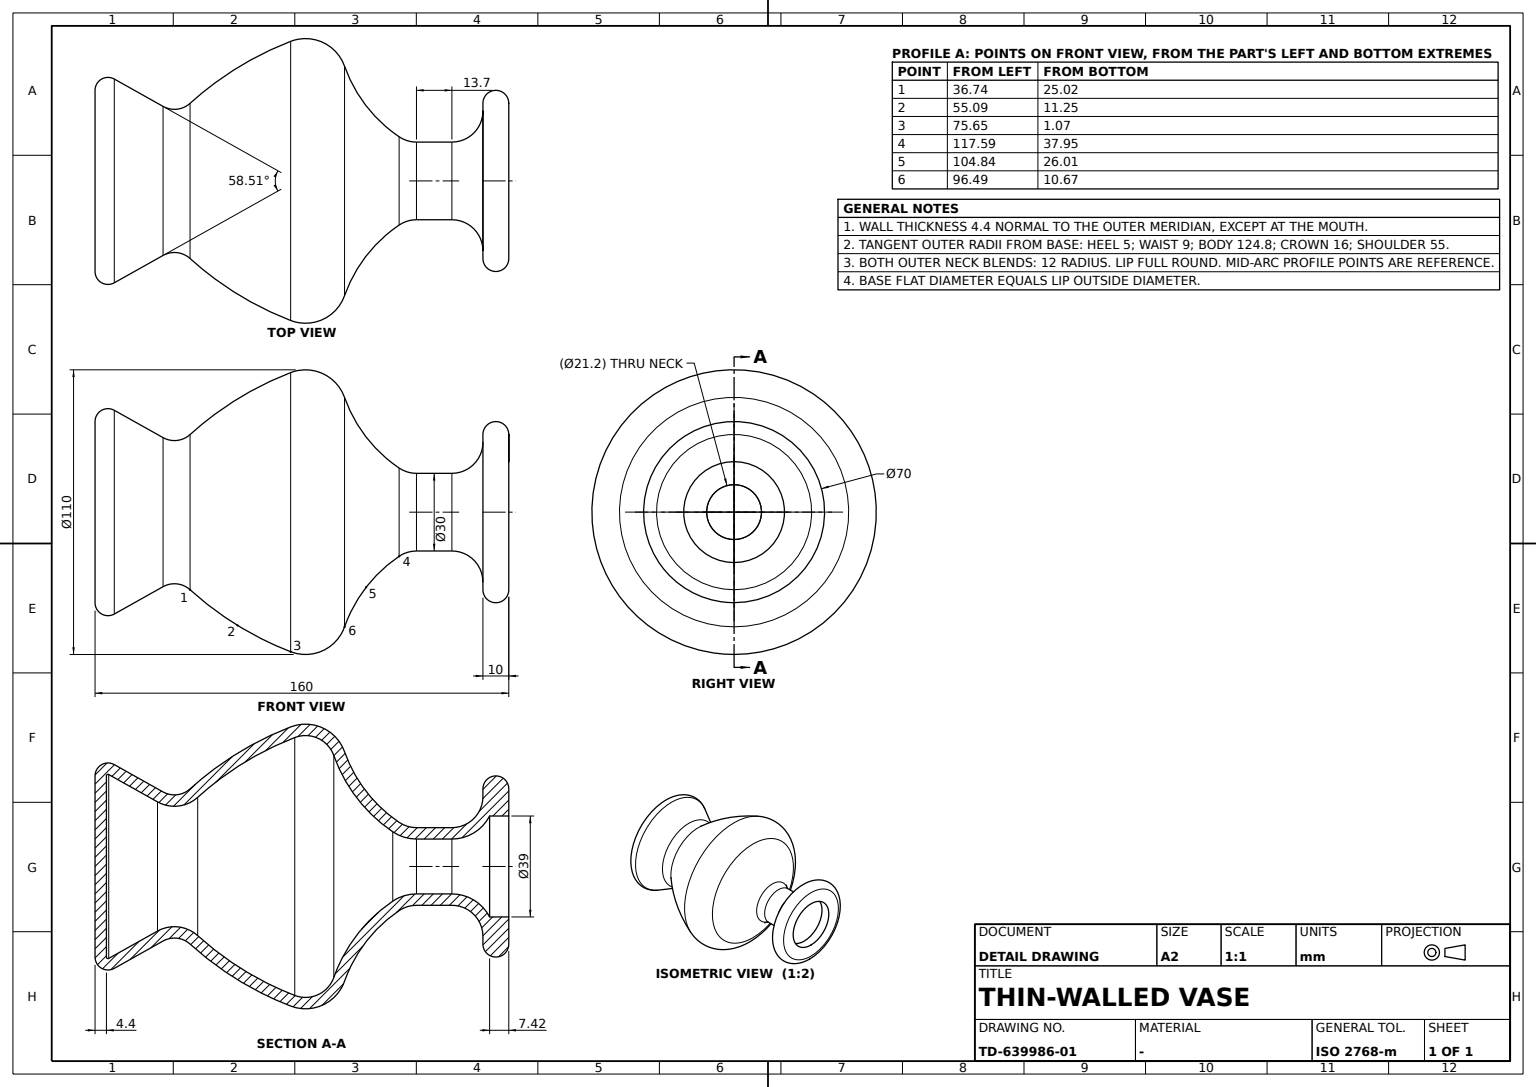
CATIA V5 part; units mm, degrees
sketch "Sketch1" plane through (0, 0, 0) normal (0, 1, 0) x (-1, 0, 0)
  line L0 (0, 0) -> (35, 0)
  arc A0 (35, 0) -> (39.3622, 7.4437) centre (35, 5) ccw
  point P0 (35, 5)
  line L1 (39.3622, 7.4437) -> (28.7981, 26.3014)
  arc A1 (28.7981, 26.3014) -> (29.979, 36.7413) centre (36.65, 30.7) cw
  point P1 (36.65, 30.7)
  point P2 (29.979, 36.7413)
  arc A2 (29.979, 36.7413) -> (53.9303, 75.6479) centre (-62.526, 120.514) ccw
  point P3 (-62.526, 120.514)
  point P4 (29.979, 36.7413)
  arc A3 (53.9303, 75.6479) -> (44.3292, 96.4864) centre (39, 81.4) ccw
  point P5 (39, 81.4)
  arc A4 (44.3292, 96.4864) -> (17.0517, 117.5895) centre (62.6481, 148.346) cw
  point P6 (62.6481, 148.346)
  arc A5 (17.0517, 117.5895) -> (15, 124.3) centre (27, 124.3) cw
  point P7 (27, 124.3)
  point P8 (15, 124.3)
  point P9 (15, 124.3)
  line L2 (15, 124.3) -> (15, 138)
  point P10 (15, 138)
  arc A6 (15, 138) -> (27, 150) centre (27, 138) cw
  point P11 (27, 138)
  line L3 (0, 155) -> (30, 155) construction
  point P12 (0, 155)
  line L4 (30, 150) -> (27, 150)
  arc A7 (30, 160) -> (30, 150) centre (30, 155) cw
  point P13 (0, 160)
  line L5 (0, 160) -> (0, 160) construction
  line L6 (0, 0) -> (0, 155) construction
  line L7 (0, 4.4) -> (35, 4.4)
  line L8 (0, 0) -> (0, 4.4) construction
  line L9 (35, 0) -> (35, 4.4) construction
  arc A8 (35, 4.4) -> (35.5235, 5.2932) centre (35, 5) ccw
  line L10 (35, 0) -> (35, 4.4) construction
  line L11 (39.3622, 7.4437) -> (35.5235, 5.2932) construction
  line L12 (35.5235, 5.2932) -> (24.9594, 24.151)
  line L13 (39.3622, 7.4437) -> (35.5235, 5.2932) construction
  line L14 (28.7981, 26.3014) -> (24.9594, 24.151) construction
  arc A9 (26.7176, 39.6948) -> (24.9594, 24.151) centre (36.65, 30.7) ccw
  line L15 (29.979, 36.7413) -> (26.7176, 39.6948) construction
  line L16 (28.7981, 26.3014) -> (24.9594, 24.151) construction
  arc A10 (26.7176, 39.6948) -> (49.8245, 77.2298) centre (-62.526, 120.514) ccw
  line L17 (29.979, 36.7413) -> (26.7176, 39.6948) construction
  line L18 (53.9303, 75.6479) -> (49.8245, 77.2298) construction
  arc A11 (49.8245, 77.2298) -> (42.8636, 92.3377) centre (39, 81.4) ccw
  line L19 (53.9303, 75.6479) -> (49.8245, 77.2298) construction
  line L20 (44.3292, 96.4864) -> (42.8636, 92.3377) construction
  arc A12 (13.404, 115.129) -> (42.8636, 92.3377) centre (62.6481, 148.346) ccw
  line L21 (17.0517, 117.5895) -> (13.404, 115.129) construction
  line L22 (44.3292, 96.4864) -> (42.8636, 92.3377) construction
  arc A13 (10.6, 124.3) -> (13.404, 115.129) centre (27, 124.3) ccw
  line L23 (15, 124.3) -> (10.6, 124.3) construction
  line L24 (17.0517, 117.5895) -> (13.404, 115.129) construction
  line L25 (10.6, 124.3) -> (10.6, 138)
  line L26 (15, 124.3) -> (10.6, 124.3) construction
  line L27 (15, 138) -> (10.6, 138) construction
  arc A14 (19.5, 152.5846) -> (10.6, 138) centre (27, 138) ccw
  line L28 (27, 150) -> (27, 154.4) construction
  line L29 (15, 138) -> (10.6, 138) construction
  line L30 (0, 160) -> (19.5, 160) construction
  point P14 (19.5, 160)
  line L31 (19.5, 160) -> (30, 160)
  line L32 (19.5, 160) -> (19.5, 152.5846)
  line L33 (0, 0) -> (0, 4.4)
  dimension "radius A0" = 5
  dimension "radius A1" = 9
  dimension "distance A1 y axis" = 27.65
  dimension "length L0" = 35
  dimension "distance A1 L0" = 21.7
  dimension "radius A2" = 124.8
  dimension "radius A3" = 16
  dimension "distance P5 A1 y axis" = 59.7
  dimension "distance A3 y axis" = 55
  dimension "length L2" = 13.7
  dimension "radius A5" = 12
  dimension "radius A4" = 55
  dimension "distance y axis P10" = 15
  dimension "radius A6" = 12
  dimension "distance A7 L5" = 35
  dimension "radius A7" = 5
  dimension "distance L0 L7" = 4.4
  dimension "distance A0 A8" = 4.4
  dimension "distance L1 L12" = 4.4
  dimension "distance A1 A9" = 4.4
  dimension "distance A2 A10" = 4.4
  dimension "distance A3 A11" = 4.4
  dimension "distance A4 A12" = 4.4
  dimension "distance A5 A13" = 4.4
  dimension "distance L2 L25" = 4.4
  dimension "distance A6 A14" = 4.4
  dimension "distance A7 P14 x axis" = 15.5
  dimension "distance L31 L0" = 160
  constraint horizontal L0 x-axis
  constraint horizontal L3 x-axis
  constraint horizontal L4 x-axis
  constraint horizontal L31 x-axis
  constraint tangency A0 L0
  constraint tangency L1 A0
  constraint tangency A1 L1
  constraint tangency A3 A2
  constraint tangency A2 A1
  constraint tangency A5 L2
  constraint tangency A4 A3
  constraint tangency A4 A5
  constraint tangency A6 L2
  constraint tangency A7 L4
  constraint tangency A6 L4
  constraint tangency L30 A7
  constraint tangency L31 A7
  constraint coincidence P2 P4
  constraint coincidence P9 A5
  constraint coincidence P9 P8
  constraint coincidence P12 y-axis
  constraint coincidence P13 L5
  constraint coincidence P13 y-axis
  constraint coincidence L10 P0
  constraint coincidence L11 P0
  constraint coincidence L15 P1
  constraint coincidence L16 P1
  constraint coincidence L17 P3
  constraint coincidence L18 P3
  constraint coincidence L19 P5
  constraint coincidence L20 P5
  constraint coincidence L21 P6
  constraint coincidence L22 P6
  constraint coincidence L23 P7
  constraint coincidence L24 P7
  constraint coincidence L28 P11
  constraint coincidence L29 P11
  constraint vertical L2 y-axis
  constraint vertical L5 y-axis
  constraint vertical L6 y-axis
  constraint vertical L32 y-axis
  constraint vertical L33 y-axis
  constraint perpendicularity L8 L0
  constraint perpendicularity L8 L7
  constraint perpendicularity L9 L0
  constraint perpendicularity L9 L7
  constraint perpendicularity L13 L1
  constraint perpendicularity L13 L12
  constraint perpendicularity L14 L1
  constraint perpendicularity L14 L12
  constraint perpendicularity L26 L2
  constraint perpendicularity L26 L25
  constraint perpendicularity L27 L2
  constraint perpendicularity L27 L25
  constraint concentricity A0 A8
  constraint concentricity A1 A9
  constraint concentricity A2 A10
  constraint concentricity A3 A11
  constraint concentricity A4 A12
  constraint concentricity A5 A13
  constraint concentricity A6 A14
revolve "Shaft1" add sketch "Sketch1" angle 360 about axis through (0, 0, 0) along (0, 0, 1)
